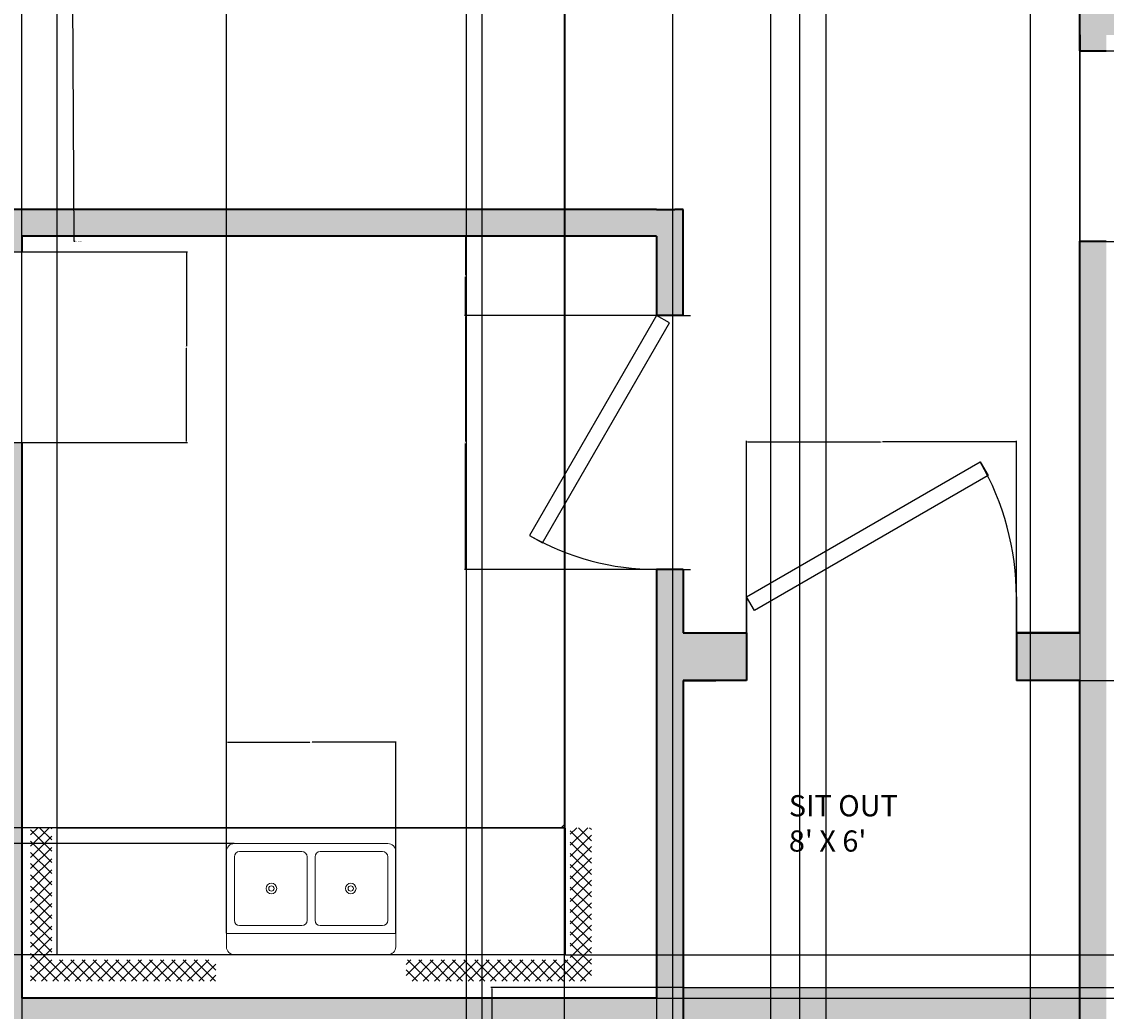
# Model space of a CAD drawing. Units: inches. Extents: x -7 to 546, y -27 to 766.
# Tile 3 of 9: x 127 to 332, y 89 to 276. Entities that reach past the tile are written whole.
import ezdxf

# ---------------------------------------------------------------- set-up
doc = ezdxf.new("R2010")
doc.units = ezdxf.units.IN
doc.header["$MEASUREMENT"] = 0
for name, color, linetype, lineweight in [('A-ANNO-DIMS', 2, 'Continuous', 18), ('A-AREA-IDEN', 7, 'Continuous', 18), ('A-FLOR-CASE-PATT', 181, 'Continuous', 13), ('A-FLOR-FIXT', 9, 'Continuous', 18), ('A-FLOR-STRS', 7, 'Continuous', 25), ('A-WALL', 7, 'Continuous', 35), ('doors', 40, 'Continuous', 25), ('kitchen', 181, 'Continuous', 25)]:
    doc.layers.add(name, color=color, linetype=linetype, lineweight=lineweight)
doc.layers.add('A-FLOR-PATT', color=143, linetype='Continuous', lineweight=13, true_color=0x7aafdf)
doc.layers.add('A-WALL-PATT', color=251, linetype='Continuous', lineweight=13, true_color=0x636466)
doc.styles.get("Standard").update_dxf_attribs({"font": 'arial.ttf'})
doc.dimstyles.get("Standard").update_dxf_attribs({"dimtxt": 0.18, "dimasz": 0.18, "dimexe": 0.18, "dimexo": 0.0625, "dimgap": 0.09, "dimtad": 0, "dimtih": 1, "dimtoh": 1, "dimdec": 4, "dimzin": 0, "dimdsep": 46, "dimtxsty": 'Standard', "dimcen": 0.09, "dimadec": 0, "dimazin": 0, "dimtfac": 1, "dimtdec": 4, "dimtofl": 0, "dimtmove": 0, "dimatfit": 3, "dimfxl": 1, "dimtolj": 1, "dimtzin": 0, "dimarcsym": 0})

# ---------------------------------------------------------------- blocks, each defined once
blk = doc.blocks.new('*U11')
for p, q in [((0, 0), (0, 100)), ((750, 0), (750, 100))]:
    blk.add_line(p, q)
blk.add_lwpolyline([(0, 0), (649.5, -375), (671.4, -337.1), (21.9, 37.9)], close=True)
blk.add_arc((0, 0), 750, 330, 0)
blk = doc.blocks.new('*U10')
for p, q in [((0, 0), (0, -100)), ((750, 0), (750, -100))]:
    blk.add_line(p, q)
blk.add_lwpolyline([(0, 0), (649.5, 375), (671.4, 337.1), (21.9, -37.9)], close=True)
blk.add_arc((0, 0), 750, 0, 30)
blk = doc.blocks.new('*D39')
at = {"layer": 'A-ANNO-DIMS', "color": 0, "lineweight": -2, "transparency": 16777216}
for p, q in [((214.23, 600.68), (214.23, -26.56)), ((250.23, 600.68), (250.23, -26.56)), ((214.41, -26.38), (232.01, -26.38)), ((250.05, -26.38), (232.45, -26.38))]:
    blk.add_line(p, q, dxfattribs=at)
at = {"layer": 'A-ANNO-DIMS', "color": 0, "transparency": 16777216}
for points in [[(214.41, -26.35), (214.41, -26.41), (214.23, -26.38)], [(250.05, -26.35), (250.05, -26.41), (250.23, -26.38)]]:
    blk.add_solid(points, dxfattribs=at)
at = {"layer": 'Defpoints', "color": 0, "transparency": 16777216}
for p in [(214.23, 600.74), (250.23, 600.74), (250.23, -26.38)]:
    blk.add_point(p, dxfattribs=at)
at = {"layer": 'A-ANNO-DIMS', "color": 0, "transparency": 16777216, "insert": (232.23, -26.38), "char_height": 0.18, "attachment_point": 5}
blk.add_mtext('\\A1;36', dxfattribs=at)
blk = doc.blocks.new('*D41')
at = {"layer": 'A-ANNO-DIMS', "color": 0, "lineweight": -2, "transparency": 16777216}
for p, q in [((274.23, 600.68), (274.23, -26.56)), ((279.23, 600.68), (279.23, -26.56)), ((274.41, -26.38), (276.58, -26.38)), ((279.05, -26.38), (276.88, -26.38))]:
    blk.add_line(p, q, dxfattribs=at)
at = {"layer": 'A-ANNO-DIMS', "color": 0, "transparency": 16777216}
for points in [[(274.41, -26.35), (274.41, -26.41), (274.23, -26.38)], [(279.05, -26.35), (279.05, -26.41), (279.23, -26.38)]]:
    blk.add_solid(points, dxfattribs=at)
at = {"layer": 'Defpoints', "color": 0, "transparency": 16777216}
for p in [(274.23, 600.74), (279.23, 600.74), (279.23, -26.38)]:
    blk.add_point(p, dxfattribs=at)
at = {"layer": 'A-ANNO-DIMS', "color": 0, "transparency": 16777216, "insert": (276.73, -26.38), "char_height": 0.18, "attachment_point": 5}
blk.add_mtext('\\A1;5', dxfattribs=at)
blk = doc.blocks.new('*D42')
at = {"layer": 'A-ANNO-DIMS', "color": 0, "lineweight": -2, "transparency": 16777216}
for p, q in [((211.23, 696.68), (211.23, -26.56)), ((229.74, 696.68), (229.74, -26.56)), ((211.41, -26.38), (220.12, -26.38)), ((229.56, -26.38), (220.85, -26.38))]:
    blk.add_line(p, q, dxfattribs=at)
at = {"layer": 'A-ANNO-DIMS', "color": 0, "transparency": 16777216}
for points in [[(211.41, -26.35), (211.41, -26.41), (211.23, -26.38)], [(229.56, -26.35), (229.56, -26.41), (229.74, -26.38)]]:
    blk.add_solid(points, dxfattribs=at)
at = {"layer": 'Defpoints', "color": 0, "transparency": 16777216}
for p in [(211.23, 696.74), (229.74, 696.74), (229.74, -26.38)]:
    blk.add_point(p, dxfattribs=at)
at = {"layer": 'A-ANNO-DIMS', "color": 0, "transparency": 16777216, "insert": (220.49, -26.38), "char_height": 0.18, "attachment_point": 5}
blk.add_mtext('\\A1;18.51', dxfattribs=at)
blk = doc.blocks.new('*D43')
at = {"layer": 'A-ANNO-DIMS', "color": 0, "lineweight": -2, "transparency": 16777216}
for p, q in [((317.84, 696.68), (317.84, -26.56)), ((327.23, 696.68), (327.23, -26.56)), ((318.02, -26.38), (322.21, -26.38)), ((327.05, -26.38), (322.86, -26.38))]:
    blk.add_line(p, q, dxfattribs=at)
at = {"layer": 'A-ANNO-DIMS', "color": 0, "transparency": 16777216}
for points in [[(318.02, -26.35), (318.02, -26.41), (317.84, -26.38)], [(327.05, -26.35), (327.05, -26.41), (327.23, -26.38)]]:
    blk.add_solid(points, dxfattribs=at)
at = {"layer": 'Defpoints', "color": 0, "transparency": 16777216}
for p in [(317.84, 696.74), (327.23, 696.74), (327.23, -26.38)]:
    blk.add_point(p, dxfattribs=at)
at = {"layer": 'A-ANNO-DIMS', "color": 0, "transparency": 16777216, "insert": (322.54, -26.38), "char_height": 0.18, "attachment_point": 5}
blk.add_mtext('\\A1;9.39', dxfattribs=at)
blk = doc.blocks.new('*D45')
at = {"layer": 'A-ANNO-DIMS', "color": 0, "lineweight": -2, "transparency": 16777216}
for p, q in [((211.23, 600.68), (211.23, -26.56)), ((214.23, 600.68), (214.23, -26.56)), ((211.41, -26.38), (212.58, -26.38)), ((214.05, -26.38), (212.88, -26.38))]:
    blk.add_line(p, q, dxfattribs=at)
at = {"layer": 'A-ANNO-DIMS', "color": 0, "transparency": 16777216}
for points in [[(211.41, -26.35), (211.41, -26.41), (211.23, -26.38)], [(214.05, -26.35), (214.05, -26.41), (214.23, -26.38)]]:
    blk.add_solid(points, dxfattribs=at)
at = {"layer": 'Defpoints', "color": 0, "transparency": 16777216}
for p in [(211.23, 600.74), (214.23, 600.74), (214.23, -26.38)]:
    blk.add_point(p, dxfattribs=at)
at = {"layer": 'A-ANNO-DIMS', "color": 0, "transparency": 16777216, "insert": (212.73, -26.38), "char_height": 0.18, "attachment_point": 5}
blk.add_mtext('\\A1;3', dxfattribs=at)
blk = doc.blocks.new('*D49')
at = {"layer": 'A-ANNO-DIMS', "color": 0, "lineweight": -2, "transparency": 16777216}
for p, q in [((127.23, 91.68), (127.23, -26.56)), ((247.23, 91.68), (247.23, -26.56)), ((127.41, -26.38), (186.95, -26.38)), ((247.05, -26.38), (187.51, -26.38))]:
    blk.add_line(p, q, dxfattribs=at)
at = {"layer": 'A-ANNO-DIMS', "color": 0, "transparency": 16777216}
for points in [[(127.41, -26.35), (127.41, -26.41), (127.23, -26.38)], [(247.05, -26.35), (247.05, -26.41), (247.23, -26.38)]]:
    blk.add_solid(points, dxfattribs=at)
at = {"layer": 'Defpoints', "color": 0, "transparency": 16777216}
for p in [(127.23, 91.74), (247.23, 91.74), (247.23, -26.38)]:
    blk.add_point(p, dxfattribs=at)
at = {"layer": 'A-ANNO-DIMS', "color": 0, "transparency": 16777216, "insert": (187.23, -26.38), "char_height": 0.18, "attachment_point": 5}
blk.add_mtext('\\A1;120', dxfattribs=at)
blk = doc.blocks.new('*D51')
at = {"layer": 'A-ANNO-DIMS', "color": 0, "lineweight": -2, "transparency": 16777216}
for p, q in [((247.17, 220.74), (210.93, 220.74)), ((211.11, 220.56), (211.11, 196.93)), ((211.11, 172.92), (211.11, 196.56)), ((247.17, 172.74), (210.93, 172.74))]:
    blk.add_line(p, q, dxfattribs=at)
at = {"layer": 'A-ANNO-DIMS', "color": 0, "transparency": 16777216}
for points in [[(211.08, 220.56), (211.14, 220.56), (211.11, 220.74)], [(211.08, 172.92), (211.14, 172.92), (211.11, 172.74)]]:
    blk.add_solid(points, dxfattribs=at)
at = {"layer": 'Defpoints', "color": 0, "transparency": 16777216}
for p in [(211.11, 220.74), (247.23, 220.74), (247.23, 172.74)]:
    blk.add_point(p, dxfattribs=at)
at = {"layer": 'A-ANNO-DIMS', "color": 0, "transparency": 16777216, "insert": (211.11, 196.74), "char_height": 0.18, "attachment_point": 5}
blk.add_mtext('\\A1;48', dxfattribs=at)
blk = doc.blocks.new('*D52')
at = {"layer": 'A-ANNO-DIMS', "color": 0, "lineweight": -2, "transparency": 16777216}
for p, q in [((122.29, 232.74), (158.54, 232.74)), ((158.36, 232.56), (158.36, 214.93)), ((158.36, 196.92), (158.36, 214.56)), ((122.29, 196.74), (158.54, 196.74))]:
    blk.add_line(p, q, dxfattribs=at)
at = {"layer": 'A-ANNO-DIMS', "color": 0, "transparency": 16777216}
for points in [[(158.33, 232.56), (158.39, 232.56), (158.36, 232.74)], [(158.33, 196.92), (158.39, 196.92), (158.36, 196.74)]]:
    blk.add_solid(points, dxfattribs=at)
at = {"layer": 'Defpoints', "color": 0, "transparency": 16777216}
for p in [(122.23, 232.74), (122.23, 196.74), (158.36, 196.74)]:
    blk.add_point(p, dxfattribs=at)
at = {"layer": 'A-ANNO-DIMS', "color": 0, "transparency": 16777216, "insert": (158.36, 214.74), "char_height": 0.18, "attachment_point": 5}
blk.add_mtext('\\A1;36', dxfattribs=at)
blk = doc.blocks.new('*D53')
at = {"layer": 'A-ANNO-DIMS', "color": 0, "lineweight": -2, "transparency": 16777216}
for p, q in [((133.93, 124.01), (133.93, 766.05)), ((134.11, 765.87), (181.71, 765.87)), ((229.75, 765.87), (182.15, 765.87)), ((229.93, 124.01), (229.93, 766.05))]:
    blk.add_line(p, q, dxfattribs=at)
at = {"layer": 'A-ANNO-DIMS', "color": 0, "transparency": 16777216}
for points in [[(134.11, 765.9), (134.11, 765.84), (133.93, 765.87)], [(229.75, 765.9), (229.75, 765.84), (229.93, 765.87)]]:
    blk.add_solid(points, dxfattribs=at)
at = {"layer": 'Defpoints', "color": 0, "transparency": 16777216}
for p in [(229.93, 765.87), (133.93, 123.94), (229.93, 123.94)]:
    blk.add_point(p, dxfattribs=at)
at = {"layer": 'A-ANNO-DIMS', "color": 0, "transparency": 16777216, "insert": (181.93, 765.87), "char_height": 0.18, "attachment_point": 5}
blk.add_mtext('\\A1;96', dxfattribs=at)
blk = doc.blocks.new('*D54')
at = {"layer": 'A-ANNO-DIMS', "color": 0, "lineweight": -2, "transparency": 16777216}
for p, q in [((229.86, 123.94), (-7.07, 123.94)), ((-6.89, 123.76), (-6.89, 112.12)), ((-6.89, 100.12), (-6.89, 111.76)), ((229.86, 99.94), (-7.07, 99.94))]:
    blk.add_line(p, q, dxfattribs=at)
at = {"layer": 'A-ANNO-DIMS', "color": 0, "transparency": 16777216}
for points in [[(-6.92, 123.76), (-6.86, 123.76), (-6.89, 123.94)], [(-6.92, 100.12), (-6.86, 100.12), (-6.89, 99.94)]]:
    blk.add_solid(points, dxfattribs=at)
at = {"layer": 'Defpoints', "color": 0, "transparency": 16777216}
for p in [(229.93, 123.94), (-6.89, 99.94), (229.93, 99.94)]:
    blk.add_point(p, dxfattribs=at)
at = {"layer": 'A-ANNO-DIMS', "color": 0, "transparency": 16777216, "insert": (-6.89, 111.94), "char_height": 0.18, "attachment_point": 5}
blk.add_mtext('\\A1;24', dxfattribs=at)
blk = doc.blocks.new('*D56')
at = {"layer": 'A-ANNO-DIMS', "color": 0, "lineweight": -2, "transparency": 16777216}
for p, q in [((264.23, 160.81), (264.23, 197.05)), ((264.41, 196.87), (289.53, 196.87)), ((315.05, 196.87), (289.93, 196.87)), ((315.23, 160.81), (315.23, 197.05))]:
    blk.add_line(p, q, dxfattribs=at)
at = {"layer": 'A-ANNO-DIMS', "color": 0, "transparency": 16777216}
for points in [[(264.41, 196.9), (264.41, 196.84), (264.23, 196.87)], [(315.05, 196.9), (315.05, 196.84), (315.23, 196.87)]]:
    blk.add_solid(points, dxfattribs=at)
at = {"layer": 'Defpoints', "color": 0, "transparency": 16777216}
for p in [(315.23, 196.87), (264.23, 160.74), (315.23, 160.74)]:
    blk.add_point(p, dxfattribs=at)
at = {"layer": 'A-ANNO-DIMS', "color": 0, "transparency": 16777216, "insert": (289.73, 196.87), "char_height": 0.18, "attachment_point": 5}
blk.add_mtext('\\A1;51', dxfattribs=at)
blk = doc.blocks.new('*D59')
at = {"layer": 'A-ANNO-DIMS', "color": 0, "lineweight": -2, "transparency": 16777216}
for p, q in [((327.29, 151.74), (363.54, 151.74)), ((363.36, 151.56), (363.36, 122.93)), ((363.36, 93.92), (363.36, 122.56)), ((327.29, 93.74), (363.54, 93.74))]:
    blk.add_line(p, q, dxfattribs=at)
at = {"layer": 'A-ANNO-DIMS', "color": 0, "transparency": 16777216}
for points in [[(363.33, 151.56), (363.39, 151.56), (363.36, 151.74)], [(363.33, 93.92), (363.39, 93.92), (363.36, 93.74)]]:
    blk.add_solid(points, dxfattribs=at)
at = {"layer": 'Defpoints', "color": 0, "transparency": 16777216}
for p in [(327.23, 151.74), (327.23, 93.74), (363.36, 93.74)]:
    blk.add_point(p, dxfattribs=at)
at = {"layer": 'A-ANNO-DIMS', "color": 0, "transparency": 16777216, "insert": (363.36, 122.74), "char_height": 0.18, "attachment_point": 5}
blk.add_mtext('\\A1;58', dxfattribs=at)
blk = doc.blocks.new('*D60')
at = {"layer": 'A-ANNO-DIMS', "color": 0, "lineweight": -2, "transparency": 16777216}
for p, q in [((327.29, 270.74), (363.54, 270.74)), ((363.36, 270.56), (363.36, 252.93)), ((363.36, 234.92), (363.36, 252.56)), ((327.29, 234.74), (363.54, 234.74))]:
    blk.add_line(p, q, dxfattribs=at)
at = {"layer": 'A-ANNO-DIMS', "color": 0, "transparency": 16777216}
for points in [[(363.33, 270.56), (363.39, 270.56), (363.36, 270.74)], [(363.33, 234.92), (363.39, 234.92), (363.36, 234.74)]]:
    blk.add_solid(points, dxfattribs=at)
at = {"layer": 'Defpoints', "color": 0, "transparency": 16777216}
for p in [(327.23, 270.74), (327.23, 234.74), (363.36, 234.74)]:
    blk.add_point(p, dxfattribs=at)
at = {"layer": 'A-ANNO-DIMS', "color": 0, "transparency": 16777216, "insert": (363.36, 252.74), "char_height": 0.18, "attachment_point": 5}
blk.add_mtext('\\A1;36', dxfattribs=at)
blk = doc.blocks.new('*D66')
at = {"layer": 'A-ANNO-DIMS', "color": 0, "lineweight": -2, "transparency": 16777216}
for p, q in [((252.17, 93.74), (215.93, 93.74)), ((216.11, 93.56), (216.11, 53.93)), ((216.11, 13.92), (216.11, 53.56)), ((252.17, 13.74), (215.93, 13.74))]:
    blk.add_line(p, q, dxfattribs=at)
at = {"layer": 'A-ANNO-DIMS', "color": 0, "transparency": 16777216}
for points in [[(216.08, 93.56), (216.14, 93.56), (216.11, 93.74)], [(216.08, 13.92), (216.14, 13.92), (216.11, 13.74)]]:
    blk.add_solid(points, dxfattribs=at)
at = {"layer": 'Defpoints', "color": 0, "transparency": 16777216}
for p in [(216.11, 93.74), (252.23, 93.74), (252.23, 13.74)]:
    blk.add_point(p, dxfattribs=at)
at = {"layer": 'A-ANNO-DIMS', "color": 0, "transparency": 16777216, "insert": (216.11, 53.74), "char_height": 0.18, "attachment_point": 5}
blk.add_mtext('\\A1;80', dxfattribs=at)
blk = doc.blocks.new('*D67')
at = {"layer": 'A-ANNO-DIMS', "color": 0, "lineweight": -2, "transparency": 16777216}
for p, q in [((165.93, 104.01), (165.93, 140.25)), ((166.11, 140.07), (181.71, 140.07)), ((197.75, 140.07), (182.15, 140.07)), ((197.93, 104.01), (197.93, 140.25))]:
    blk.add_line(p, q, dxfattribs=at)
at = {"layer": 'A-ANNO-DIMS', "color": 0, "transparency": 16777216}
for points in [[(166.11, 140.1), (166.11, 140.04), (165.93, 140.07)], [(197.75, 140.1), (197.75, 140.04), (197.93, 140.07)]]:
    blk.add_solid(points, dxfattribs=at)
at = {"layer": 'Defpoints', "color": 0, "transparency": 16777216}
for p in [(197.93, 140.07), (165.93, 103.94), (197.93, 103.94)]:
    blk.add_point(p, dxfattribs=at)
at = {"layer": 'A-ANNO-DIMS', "color": 0, "transparency": 16777216, "insert": (181.93, 140.07), "char_height": 0.18, "attachment_point": 5}
blk.add_mtext('\\A1;32', dxfattribs=at)
blk = doc.blocks.new('*D68')
at = {"layer": 'A-ANNO-DIMS', "color": 0, "lineweight": -2, "transparency": 16777216}
for p, q in [((133.93, 100.01), (133.93, 766.05)), ((134.11, 765.87), (149.71, 765.87)), ((165.75, 765.87), (150.15, 765.87)), ((165.93, 104.01), (165.93, 766.05))]:
    blk.add_line(p, q, dxfattribs=at)
at = {"layer": 'A-ANNO-DIMS', "color": 0, "transparency": 16777216}
for points in [[(134.11, 765.9), (134.11, 765.84), (133.93, 765.87)], [(165.75, 765.9), (165.75, 765.84), (165.93, 765.87)]]:
    blk.add_solid(points, dxfattribs=at)
at = {"layer": 'Defpoints', "color": 0, "transparency": 16777216}
for p in [(165.93, 765.87), (165.93, 103.94), (133.93, 99.94)]:
    blk.add_point(p, dxfattribs=at)
at = {"layer": 'A-ANNO-DIMS', "color": 0, "transparency": 16777216, "insert": (149.93, 765.87), "char_height": 0.18, "attachment_point": 5}
blk.add_mtext('\\A1;32', dxfattribs=at)
blk = doc.blocks.new('*D69')
at = {"layer": 'A-ANNO-DIMS', "color": 0, "lineweight": -2, "transparency": 16777216}
for p, q in [((167.36, 120.94), (-7.07, 120.94)), ((-6.89, 120.76), (-6.89, 110.62)), ((-6.89, 100.12), (-6.89, 110.26)), ((167.36, 99.94), (-7.07, 99.94))]:
    blk.add_line(p, q, dxfattribs=at)
at = {"layer": 'A-ANNO-DIMS', "color": 0, "transparency": 16777216}
for points in [[(-6.92, 120.76), (-6.86, 120.76), (-6.89, 120.94)], [(-6.92, 100.12), (-6.86, 100.12), (-6.89, 99.94)]]:
    blk.add_solid(points, dxfattribs=at)
at = {"layer": 'Defpoints', "color": 0, "transparency": 16777216}
for p in [(-6.89, 120.94), (167.43, 120.94), (167.43, 99.94)]:
    blk.add_point(p, dxfattribs=at)
at = {"layer": 'A-ANNO-DIMS', "color": 0, "transparency": 16777216, "insert": (-6.89, 110.44), "char_height": 0.18, "attachment_point": 5}
blk.add_mtext('\\A1;21', dxfattribs=at)
blk = doc.blocks.new('*D80')
at = {"layer": 'A-ANNO-DIMS', "color": 0, "lineweight": -2, "transparency": 16777216}
for p, q in [((247.17, 235.74), (210.93, 235.74)), ((211.11, 235.56), (211.11, 228.43)), ((211.11, 220.92), (211.11, 228.06)), ((247.17, 220.74), (210.93, 220.74))]:
    blk.add_line(p, q, dxfattribs=at)
at = {"layer": 'A-ANNO-DIMS', "color": 0, "transparency": 16777216}
for points in [[(211.08, 235.56), (211.14, 235.56), (211.11, 235.74)], [(211.08, 220.92), (211.14, 220.92), (211.11, 220.74)]]:
    blk.add_solid(points, dxfattribs=at)
at = {"layer": 'Defpoints', "color": 0, "transparency": 16777216}
for p in [(211.11, 235.74), (247.23, 235.74), (247.23, 220.74)]:
    blk.add_point(p, dxfattribs=at)
at = {"layer": 'A-ANNO-DIMS', "color": 0, "transparency": 16777216, "insert": (211.11, 228.24), "char_height": 0.18, "attachment_point": 5}
blk.add_mtext('\\A1;15', dxfattribs=at)
blk = doc.blocks.new('*D81')
at = {"layer": 'A-ANNO-DIMS', "color": 0, "lineweight": -2, "transparency": 16777216}
for p, q in [((62.23, 240.81), (62.23, 766.05)), ((62.41, 765.87), (194.44, 765.87)), ((327.05, 765.87), (195.02, 765.87)), ((327.23, 234.81), (327.23, 766.05))]:
    blk.add_line(p, q, dxfattribs=at)
at = {"layer": 'A-ANNO-DIMS', "color": 0, "transparency": 16777216}
for points in [[(62.41, 765.9), (62.41, 765.84), (62.23, 765.87)], [(327.05, 765.9), (327.05, 765.84), (327.23, 765.87)]]:
    blk.add_solid(points, dxfattribs=at)
at = {"layer": 'Defpoints', "color": 0, "transparency": 16777216}
for p in [(327.23, 765.87), (62.23, 240.74), (327.23, 234.74)]:
    blk.add_point(p, dxfattribs=at)
at = {"layer": 'A-ANNO-DIMS', "color": 0, "transparency": 16777216, "insert": (194.73, 765.87), "char_height": 0.18, "attachment_point": 5}
blk.add_mtext('\\A1;265', dxfattribs=at)
blk = doc.blocks.new('*D83')
at = {"layer": 'A-ANNO-DIMS', "color": 0, "lineweight": -2, "transparency": 16777216}
for p, q in [((127.23, 91.81), (127.23, 766.05)), ((127.41, 765.87), (130.18, 765.87)), ((133.75, 765.87), (130.97, 765.87)), ((133.93, 100.01), (133.93, 766.05))]:
    blk.add_line(p, q, dxfattribs=at)
at = {"layer": 'A-ANNO-DIMS', "color": 0, "transparency": 16777216}
for points in [[(127.41, 765.9), (127.41, 765.84), (127.23, 765.87)], [(133.75, 765.9), (133.75, 765.84), (133.93, 765.87)]]:
    blk.add_solid(points, dxfattribs=at)
at = {"layer": 'Defpoints', "color": 0, "transparency": 16777216}
for p in [(133.93, 765.87), (133.93, 99.94), (127.23, 91.74)]:
    blk.add_point(p, dxfattribs=at)
at = {"layer": 'A-ANNO-DIMS', "color": 0, "transparency": 16777216, "insert": (130.58, 765.87), "char_height": 0.18, "attachment_point": 5}
blk.add_mtext('\\A1;6.695', dxfattribs=at)
blk = doc.blocks.new('*D84')
at = {"layer": 'A-ANNO-DIMS', "color": 0, "lineweight": -2, "transparency": 16777216}
for p, q in [((229.99, 99.94), (545.54, 99.94)), ((545.36, 99.76), (545.36, 96.03)), ((545.36, 91.92), (545.36, 95.66)), ((247.29, 91.74), (545.54, 91.74))]:
    blk.add_line(p, q, dxfattribs=at)
at = {"layer": 'A-ANNO-DIMS', "color": 0, "transparency": 16777216}
for points in [[(545.33, 99.76), (545.39, 99.76), (545.36, 99.94)], [(545.33, 91.92), (545.39, 91.92), (545.36, 91.74)]]:
    blk.add_solid(points, dxfattribs=at)
at = {"layer": 'Defpoints', "color": 0, "transparency": 16777216}
for p in [(229.93, 99.94), (545.36, 99.94), (247.23, 91.74)]:
    blk.add_point(p, dxfattribs=at)
at = {"layer": 'A-ANNO-DIMS', "color": 0, "transparency": 16777216, "insert": (545.36, 95.84), "char_height": 0.18, "attachment_point": 5}
blk.add_mtext('\\A1;8.199', dxfattribs=at)
blk = doc.blocks.new('*D85')
at = {"layer": 'A-ANNO-DIMS', "color": 0, "lineweight": -2, "transparency": 16777216}
for p, q in [((274.23, 696.68), (274.23, -26.56)), ((268.74, 692.17), (268.74, -26.56)), ((268.92, -26.38), (271.09, -26.38)), ((274.05, -26.38), (271.88, -26.38))]:
    blk.add_line(p, q, dxfattribs=at)
at = {"layer": 'A-ANNO-DIMS', "color": 0, "transparency": 16777216}
for points in [[(268.92, -26.35), (268.92, -26.41), (268.74, -26.38)], [(274.05, -26.35), (274.05, -26.41), (274.23, -26.38)]]:
    blk.add_solid(points, dxfattribs=at)
at = {"layer": 'Defpoints', "color": 0, "transparency": 16777216}
for p in [(274.23, 696.74), (268.74, 692.23), (268.74, -26.38)]:
    blk.add_point(p, dxfattribs=at)
at = {"layer": 'A-ANNO-DIMS', "color": 0, "transparency": 16777216, "insert": (271.49, -26.38), "char_height": 0.18, "attachment_point": 5}
blk.add_mtext('\\A1;5.493', dxfattribs=at)
blk = doc.blocks.new('*D90')
at = {"layer": 'A-ANNO-DIMS', "color": 0, "lineweight": -2, "transparency": 16777216}
for p, q in [((136.15, 417.53), (136.33, 417.53)), ((136.24, 417.44), (136.24, 417.62)), ((137.16, 234.74), (136.81, 303.11)), ((137.34, 234.74), (137.16, 234.74))]:
    blk.add_line(p, q, dxfattribs=at)
at = {"layer": 'A-ANNO-DIMS', "color": 0, "transparency": 16777216}
blk.add_solid([(136.84, 303.11), (136.78, 303.11), (136.81, 303.29)], dxfattribs=at)
at = {"layer": 'Defpoints', "color": 0, "transparency": 16777216}
for p in [(136.24, 417.53), (136.81, 303.29)]:
    blk.add_point(p, dxfattribs=at)
at = {"layer": 'A-ANNO-DIMS', "color": 0, "transparency": 16777216, "insert": (138.08, 234.74), "char_height": 0.18, "attachment_point": 5}
blk.add_mtext('\\A1;3X R114.25', dxfattribs=at)

msp = doc.modelspace()

# ---------------------------------------------------------------- hatches: boundary and pattern name
at = {"layer": 'A-FLOR-CASE-PATT'}
h = msp.add_hatch(dxfattribs=at)
h.set_pattern_fill('ANSI37', color=256, scale=12, style=0)
h.paths.add_polyline_path([(128.9271, 94.9426), (163.9271, 94.9426), (163.9271, 98.9426), (132.9271, 98.9426), (132.9271, 123.9426), (128.9271, 123.9426)])
h = msp.add_hatch(dxfattribs=at)
h.set_pattern_fill('ANSI37', color=256, scale=12, style=0)
h.paths.add_polyline_path([(199.9271, 94.9426), (234.9271, 94.9426), (234.9271, 123.9426), (230.9271, 123.9426), (230.9271, 98.9426), (199.9271, 98.9426)])
at = {"layer": 'A-FLOR-PATT'}
h = msp.add_hatch(color=256, dxfattribs=at)
h.dxf.hatch_style = 1
h.paths.add_polyline_path([(327.2319, 93.744), (252.2319, 93.744), (252.2319, 83.744), (327.2319, 83.744)])
h.paths.add_polyline_path([(327.2319, 83.744), (252.2319, 83.744), (252.2319, 73.744), (327.2319, 73.744)])
h.paths.add_polyline_path([(327.2319, 73.744), (252.2319, 73.744), (252.2319, 63.744), (327.2319, 63.744)])
h.paths.add_polyline_path([(327.2319, 63.744), (252.2319, 63.744), (252.2319, 53.744), (327.2319, 53.744)])
h.paths.add_polyline_path([(327.2319, 53.744), (252.2319, 53.744), (252.2319, 43.744), (327.2319, 43.744)])
h.paths.add_polyline_path([(327.2319, 43.744), (252.2319, 43.744), (252.2319, 33.744), (327.2319, 33.744)])
h.paths.add_polyline_path([(327.2319, 33.744), (252.2319, 33.744), (252.2319, 23.744), (327.2319, 23.744)])
h.paths.add_polyline_path([(327.2319, 23.744), (252.2319, 23.744), (252.2319, 13.744), (327.2319, 13.744)])
at = {"layer": 'A-WALL-PATT'}
h = msp.add_hatch(color=256, dxfattribs=at)
h.dxf.hatch_style = 1
h.paths.add_polyline_path([(62.2319, 696.744), (86.6896, 696.744), (86.6896, 705.744), (53.2319, 705.744), (53.2319, 627.8642), (57.7271, 627.8642), (62.2319, 627.8642)])
h.paths.add_polyline_path([(229.7414, 705.744), (134.6896, 705.744), (134.6896, 696.744), (206.2319, 696.744), (206.2319, 567.744), (211.2319, 567.744), (211.2319, 595.744), (214.2319, 595.744), (214.2319, 600.744), (211.2319, 600.744), (211.2319, 696.744), (229.7414, 696.744)])
h.paths.add_polyline_path([(293.8423, 705.744), (253.7414, 705.744), (253.7414, 696.744), (274.2319, 696.744), (274.2319, 600.744), (279.2319, 600.744), (279.2319, 696.744), (293.8423, 696.744)])
h.paths.add_polyline_path([(393.9743, 705.744), (317.8423, 705.744), (317.8423, 696.744), (327.2319, 696.744), (327.2319, 651.744), (332.2319, 651.744), (332.2319, 696.744), (393.9743, 696.744)])
h.paths.add_polyline_path([(485.2319, 705.744), (441.9743, 705.744), (441.9743, 696.744), (476.2319, 696.744), (476.2319, 663.6898), (480.7319, 663.6898), (485.2319, 663.6898)])
h.paths.add_polyline_path([(485.2319, 615.6898), (476.2319, 615.6898), (476.2319, 528.744), (332.2319, 528.744), (332.2319, 531.744), (327.2319, 531.744), (327.2319, 523.744), (375.2319, 523.744), (375.2319, 427.744), (327.2319, 427.744), (327.2319, 419.744), (332.2319, 419.744), (332.2319, 422.744), (413.089, 422.744), (413.089, 427.744), (380.2319, 427.744), (380.2319, 523.744), (476.2319, 523.744), (476.2319, 490.9334), (485.2319, 490.9334)])
h.paths.add_polyline_path([(485.2319, 466.9334), (476.2319, 466.9334), (476.2319, 370.0932), (480.7319, 370.0932), (485.2319, 370.0932)])
h.paths.add_polyline_path([(485.2319, 322.0932), (476.2319, 322.0932), (476.2319, 278.744), (332.2319, 278.744), (332.2319, 383.744), (327.2319, 383.744), (327.2319, 273.744), (327.2319, 270.744), (332.2319, 270.744), (332.2319, 273.744), (476.2319, 273.744), (476.2319, 201.0338), (480.7319, 201.0338), (485.2319, 201.0338)])
h.paths.add_polyline_path([(485.2319, 153.0338), (476.2319, 153.0338), (476.2319, 42.744), (461.2319, 42.744), (461.2319, 33.744), (485.2319, 33.744)])
h.paths.add_polyline_path([(332.2319, 234.744), (327.2319, 234.744), (327.2319, 160.744), (315.2319, 160.744), (315.2319, 151.744), (327.2319, 151.744), (327.2319, 33.744), (332.2319, 33.744)])
h.paths.add_polyline_path([(252.2319, 151.744), (258.4464, 151.744), (264.2319, 151.744), (264.2319, 160.744), (252.2319, 160.744), (252.2319, 172.744), (247.2319, 172.744), (247.2319, 91.744), (127.2319, 91.744), (127.2319, 196.744), (122.2319, 196.744), (122.2319, 91.744), (62.2319, 91.744), (62.2319, 126.1124), (53.2319, 126.1124), (53.2319, 9.744), (62.2319, 9.744), (62.2319, 86.744), (247.2319, 86.744), (247.2319, 33.744), (252.2319, 33.744), (252.2319, 53.744)])
h.paths.add_polyline_path([(62.2319, 235.744), (122.2319, 235.744), (122.2319, 232.744), (127.2319, 232.744), (127.2319, 235.744), (247.2319, 235.744), (247.2319, 220.744), (252.2319, 220.744), (252.2319, 240.744), (250.6678, 240.744), (247.2319, 240.744), (62.2319, 240.744), (62.2319, 322.0932), (53.2319, 322.0932), (53.2319, 174.1124), (57.7271, 174.1124), (62.2319, 174.1124)])

# ---------------------------------------------------------------- linework, layer by layer
at = {"layer": 'A-FLOR-FIXT'}
for p, q in [((181.1771, 106.4426), (181.1771, 118.4426)), ((182.6771, 118.4426), (182.6771, 106.4426)), ((197.9271, 103.9426), (165.9271, 103.9426))]:
    msp.add_line(p, q, dxfattribs=at)
for points in [[(165.9271, 101.4426), (165.9271, 119.4426)], [(167.4271, 120.9426), (196.4271, 120.9426)], [(168.4271, 119.4426), (180.1771, 119.4426)], [(183.6771, 119.4426), (195.4271, 119.4426)], [(197.9271, 119.4426), (197.9271, 101.4426)], [(167.4271, 106.4426), (167.4271, 118.4426)], [(196.4271, 118.4426), (196.4271, 106.4426)], [(180.1771, 105.4426), (168.4271, 105.4426)], [(195.4271, 105.4426), (183.6771, 105.4426)], [(196.4271, 99.9426), (167.4271, 99.9426)]]:
    msp.add_lwpolyline(points, dxfattribs=at)
for centre, radius in [((174.4271, 112.4426), 1), ((174.4271, 112.4426), 0.5), ((189.4271, 112.4426), 1), ((189.4271, 112.4426), 0.5)]:
    msp.add_circle(centre, radius, dxfattribs=at)
for centre, radius, start, end in [((167.4271, 119.4426), 1.5, 90, 180), ((168.4271, 118.4426), 1, 90, 180), ((180.1771, 118.4426), 1, 0, 90), ((183.6771, 118.4426), 1, 90, 180), ((195.4271, 118.4426), 1, 0, 90), ((196.4271, 119.4426), 1.5, 0, 90), ((168.4271, 106.4426), 1, 180, 270), ((180.1771, 106.4426), 1, 270, 0), ((183.6771, 106.4426), 1, 180, 270), ((195.4271, 106.4426), 1, 270, 0), ((167.4271, 101.4426), 1.5, 180, 270), ((196.4271, 101.4426), 1.5, 270, 0)]:
    msp.add_arc(centre, radius, start, end, dxfattribs=at)
at = {"layer": 'A-FLOR-STRS'}
msp.add_line((252.2319, 93.744), (327.2319, 93.744), dxfattribs=at)
at = {"layer": 'A-WALL'}
for p, q in [((327.2319, 273.744), (327.2319, 383.744)), ((327.2319, 270.744), (327.2319, 273.744)), ((327.2319, 273.744), (327.2319, 270.744)), ((327.2319, 270.744), (332.2319, 270.744)), ((247.2319, 240.744), (62.2319, 240.744)), ((247.2319, 240.744), (250.6678, 240.744)), ((252.2319, 240.744), (250.6678, 240.744)), ((252.2319, 220.744), (252.2319, 240.744)), ((247.2319, 235.744), (127.2319, 235.744)), ((127.2319, 235.744), (127.2319, 232.744)), ((247.2319, 235.744), (247.2319, 220.744)), ((327.2319, 160.744), (327.2319, 234.744)), ((327.2319, 234.744), (332.2319, 234.744)), ((252.2319, 220.744), (247.2319, 220.744)), ((127.2319, 196.744), (127.2319, 91.744)), ((252.2319, 172.744), (247.2319, 172.744)), ((247.2319, 172.744), (247.2319, 91.744)), ((252.2319, 172.744), (252.2319, 160.744)), ((252.2319, 172.744), (252.2319, 160.744)), ((252.2319, 160.744), (264.2319, 160.744)), ((264.2319, 160.744), (264.2319, 151.744)), ((315.2319, 160.744), (327.2319, 160.744)), ((327.2319, 160.744), (315.2319, 160.744)), ((315.2319, 160.744), (315.2319, 151.744)), ((252.2319, 151.744), (252.2319, 33.744)), ((264.2319, 151.744), (252.2319, 151.744)), ((252.2319, 151.744), (258.4464, 151.744)), ((327.2319, 151.744), (315.2319, 151.744)), ((327.2319, 13.744), (327.2319, 151.744)), ((247.2319, 91.744), (127.2319, 91.744))]:
    msp.add_line(p, q, dxfattribs=at)
at = {"layer": 'kitchen'}
for p, q in [((133.9271, 123.9426), (229.9271, 123.9426)), ((133.9271, 99.9426), (133.9271, 123.9426)), ((229.1769, 123.9426), (229.9271, 124.6928)), ((229.9271, 123.9426), (229.9271, 99.9426)), ((229.9271, 99.9426), (133.9271, 99.9426))]:
    msp.add_line(p, q, dxfattribs=at)

# ---------------------------------------------------------------- block references
at = {"layer": 'doors', "xscale": 0.0640000000000017, "yscale": 0.0640000000000017, "zscale": 0.0640000000000017, "rotation": 270}
msp.add_blockref('*U11', (247.2319, 220.744), dxfattribs=at)
at = {"layer": 'doors', "xscale": 0.0680000000000018, "yscale": 0.0680000000000018, "zscale": 0.0680000000000018}
msp.add_blockref('*U10', (264.2319, 167.544), dxfattribs=at)

# ---------------------------------------------------------------- texts
at = {"layer": 'A-AREA-IDEN', "insert": (272.2287, 130.0884), "char_height": 4, "attachment_point": 1}
msp.add_mtext_dynamic_manual_height_columns("SIT OUT\\P8' X 6'", width=80.777321, gutter_width=1, heights=[0], dxfattribs=at)

# ---------------------------------------------------------------- dimensions: what is measured, and where the dimension line sits
at = {"layer": 'A-ANNO-DIMS'}
for base, p1, p2, override, picture, middle in [((327.2319, 765.869), (62.2319, 240.744), (327.2319, 234.744), {"dimdec": 0, "dimlfac": 1, "dimrnd": 0, "dimzin": 0, "dimdsep": 46, "dimlunit": 2}, '*D81', (194.7319, 765.869)), ((133.9271, 765.869), (127.2319, 91.744), (133.9271, 99.9426), {"dimdec": 3, "dimlfac": 1, "dimrnd": 0, "dimzin": 0, "dimdsep": 46, "dimlunit": 2}, '*D83', (130.5795, 765.869)), ((229.9271, 765.869), (133.9271, 123.9426), (229.9271, 123.9426), {"dimdec": 0, "dimlfac": 1, "dimrnd": 0, "dimzin": 0, "dimdsep": 46, "dimlunit": 2}, '*D53', (181.9271, 765.869)), ((165.9271, 765.869), (133.9271, 99.9426), (165.9271, 103.9426), {"dimdec": 0, "dimlfac": 1, "dimrnd": 0, "dimzin": 0, "dimdsep": 46, "dimlunit": 2}, '*D68', (149.9271, 765.869)), ((229.7414, -26.381), (211.2319, 696.744), (229.7414, 696.744), {"dimdec": 2, "dimlfac": 1, "dimrnd": 0, "dimzin": 0, "dimdsep": 46, "dimlunit": 2}, '*D42', (220.4867, -26.381)), ((268.7385, -26.381), (274.2319, 696.744), (268.7385, 692.2322), {"dimdec": 3, "dimlfac": 1, "dimrnd": 0, "dimzin": 0, "dimdsep": 46, "dimlunit": 2}, '*D85', (271.4852, -26.381)), ((327.2319, -26.381), (317.8423, 696.744), (327.2319, 696.744), {"dimdec": 2, "dimlfac": 1, "dimrnd": 0, "dimzin": 0, "dimdsep": 46, "dimlunit": 2}, '*D43', (322.5371, -26.381)), ((214.2319, -26.381), (211.2319, 600.744), (214.2319, 600.744), {"dimdec": 0, "dimlfac": 1, "dimrnd": 0, "dimzin": 0, "dimdsep": 46, "dimlunit": 2}, '*D45', (212.7319, -26.381)), ((250.2319, -26.381), (214.2319, 600.744), (250.2319, 600.744), {"dimdec": 0, "dimlfac": 1, "dimrnd": 0, "dimzin": 0, "dimdsep": 46, "dimlunit": 2}, '*D39', (232.2319, -26.381)), ((279.2319, -26.381), (274.2319, 600.744), (279.2319, 600.744), {"dimdec": 0, "dimlfac": 1, "dimrnd": 0, "dimzin": 0, "dimdsep": 46, "dimlunit": 2}, '*D41', (276.7319, -26.381)), ((315.2319, 196.869), (264.2319, 160.744), (315.2319, 160.744), {"dimdec": 0, "dimlfac": 1, "dimrnd": 0, "dimzin": 0, "dimdsep": 46, "dimlunit": 2}, '*D56', (289.7319, 196.869)), ((197.9271, 140.0676), (165.9271, 103.9426), (197.9271, 103.9426), {"dimdec": 0, "dimlfac": 1, "dimrnd": 0, "dimzin": 0, "dimdsep": 46, "dimlunit": 2}, '*D67', (181.9271, 140.0676)), ((247.2319, -26.381), (127.2319, 91.744), (247.2319, 91.744), {"dimdec": 0, "dimlfac": 1, "dimrnd": 0, "dimzin": 0, "dimdsep": 46, "dimlunit": 2}, '*D49', (187.2319, -26.381))]:
    dim = msp.add_linear_dim(base=base, p1=p1, p2=p2, dimstyle='Standard', override=override, dxfattribs=at)
    dim.commit()
    dim.dimension.update_dxf_attribs({"geometry": picture, "text_midpoint": middle})
dim = msp.add_radius_dim(center=(136.2373, 417.5348), mpoint=(136.811, 303.2863), text='3X <>', dimstyle='Standard', override={"dimdec": 2, "dimlfac": 1, "dimrnd": 0, "dimzin": 0, "dimdsep": 46, "dimlunit": 2}, dxfattribs=at)
dim.commit()
dim.dimension.update_dxf_attribs({"geometry": '*D90', "text_midpoint": (138.079, 234.7371), "dimtype": 164})
for base, p1, p2, angle, override, picture, middle in [((363.3569, 234.744), (327.2319, 270.744), (327.2319, 234.744), 270, {"dimdec": 0, "dimlfac": 1, "dimrnd": 0, "dimzin": 0, "dimdsep": 46, "dimlunit": 2}, '*D60', (363.3569, 252.744)), ((211.1069, 235.744), (247.2319, 220.744), (247.2319, 235.744), 90, {"dimdec": 0, "dimlfac": 1, "dimrnd": 0, "dimzin": 0, "dimdsep": 46, "dimlunit": 2}, '*D80', (211.1069, 228.244)), ((158.3569, 196.744), (122.2319, 232.744), (122.2319, 196.744), 270, {"dimdec": 0, "dimlfac": 1, "dimrnd": 0, "dimzin": 0, "dimdsep": 46, "dimlunit": 2}, '*D52', (158.3569, 214.744)), ((211.1069, 220.744), (247.2319, 172.744), (247.2319, 220.744), 90, {"dimdec": 0, "dimlfac": 1, "dimrnd": 0, "dimzin": 0, "dimdsep": 46, "dimlunit": 2}, '*D51', (211.1069, 196.744)), ((363.3569, 93.744), (327.2319, 151.744), (327.2319, 93.744), 270, {"dimdec": 0, "dimlfac": 1, "dimrnd": 0, "dimzin": 0, "dimdsep": 46, "dimlunit": 2}, '*D59', (363.3569, 122.744)), ((-6.8931, 99.9426), (229.9271, 123.9426), (229.9271, 99.9426), 90, {"dimdec": 0, "dimlfac": 1, "dimrnd": 0, "dimzin": 0, "dimdsep": 46, "dimlunit": 2}, '*D54', (-6.8931, 111.9426)), ((-6.8931, 120.9426), (167.4271, 99.9426), (167.4271, 120.9426), 90, {"dimdec": 0, "dimlfac": 1, "dimrnd": 0, "dimzin": 0, "dimdsep": 46, "dimlunit": 2}, '*D69', (-6.8931, 110.4426)), ((545.3569, 99.9426), (247.2319, 91.744), (229.9271, 99.9426), 90, {"dimdec": 3, "dimlfac": 1, "dimrnd": 0, "dimzin": 0, "dimdsep": 46, "dimlunit": 2}, '*D84', (545.3569, 95.8433)), ((216.1069, 93.744), (252.2319, 13.744), (252.2319, 93.744), 90, {"dimdec": 0, "dimlfac": 1, "dimrnd": 0, "dimzin": 0, "dimdsep": 46, "dimlunit": 2}, '*D66', (216.1069, 53.744))]:
    dim = msp.add_linear_dim(base=base, p1=p1, p2=p2, angle=angle, dimstyle='Standard', override=override, dxfattribs=at)
    dim.commit()
    dim.dimension.update_dxf_attribs({"geometry": picture, "text_midpoint": middle})

doc.saveas('drawing.dxf')
